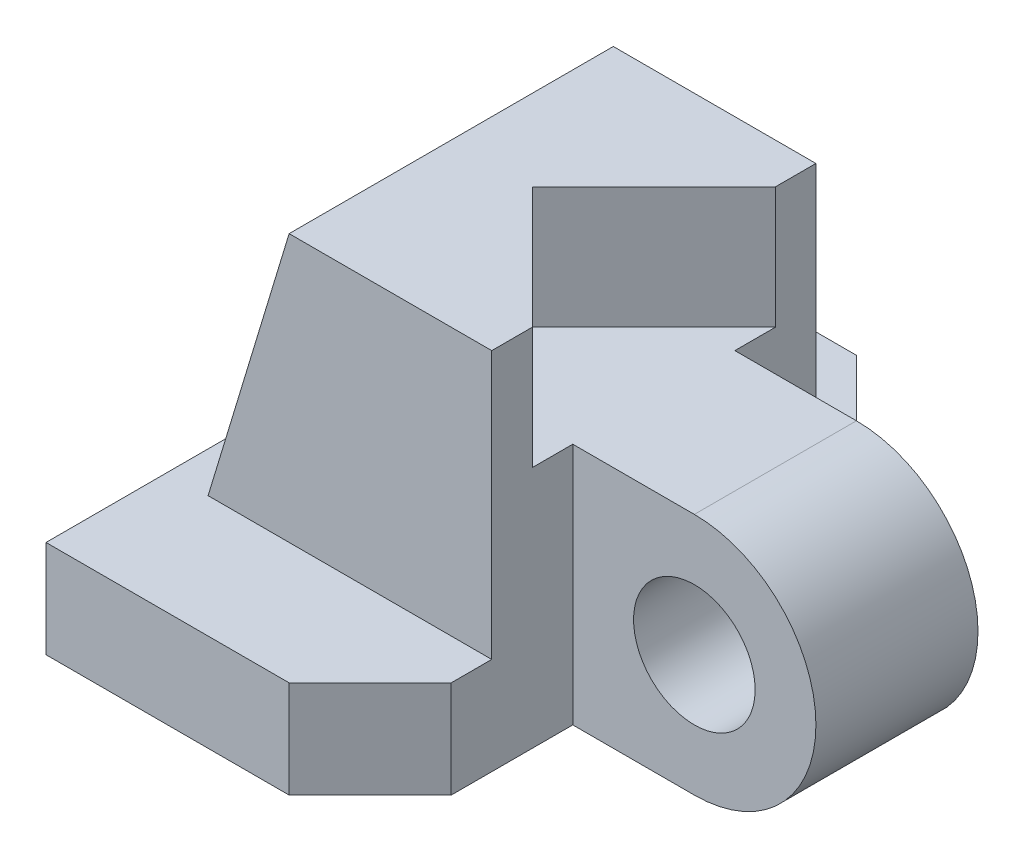
ISO-10303-21;
HEADER;
FILE_DESCRIPTION(('STEP AP214'),'2;1');
FILE_NAME('part.step','',(''),(''),'','','');
FILE_SCHEMA(('AUTOMOTIVE_DESIGN { 1 0 10303 214 1 1 1 1 }'));
ENDSEC;
DATA;
#1=APPLICATION_CONTEXT('core data for automotive mechanical design processes');
#2=APPLICATION_PROTOCOL_DEFINITION('international standard','automotive_design',2000,#1);
#3=PRODUCT_CONTEXT('',#1,'mechanical');
#4=PRODUCT('Part','Part','',(#3));
#5=PRODUCT_RELATED_PRODUCT_CATEGORY('part','',(#4));
#6=PRODUCT_DEFINITION_FORMATION('','',#4);
#7=PRODUCT_DEFINITION_CONTEXT('part definition',#1,'design');
#8=PRODUCT_DEFINITION('design','',#6,#7);
#9=PRODUCT_DEFINITION_SHAPE('','',#8);
#10=(LENGTH_UNIT() NAMED_UNIT(*) SI_UNIT(.MILLI.,.METRE.));
#11=(NAMED_UNIT(*) PLANE_ANGLE_UNIT() SI_UNIT($,.RADIAN.));
#12=(NAMED_UNIT(*) SI_UNIT($,.STERADIAN.) SOLID_ANGLE_UNIT());
#13=UNCERTAINTY_MEASURE_WITH_UNIT(LENGTH_MEASURE(1.E-05),#10,'distance_accuracy_value','');
#14=(GEOMETRIC_REPRESENTATION_CONTEXT(3) GLOBAL_UNCERTAINTY_ASSIGNED_CONTEXT((#13)) GLOBAL_UNIT_ASSIGNED_CONTEXT((#10,
#11,#12)) REPRESENTATION_CONTEXT('',''));
#15=CARTESIAN_POINT('',(0.,0.,0.));
#16=DIRECTION('',(0.,0.,1.));
#17=DIRECTION('',(1.,0.,0.));
#18=AXIS2_PLACEMENT_3D('',#15,#16,#17);
#19=CARTESIAN_POINT('',(-15.,0.,35.));
#20=DIRECTION('',(1.,0.,0.));
#21=DIRECTION('',(0.,1.,0.));
#22=AXIS2_PLACEMENT_3D('',#19,#20,#21);
#23=PLANE('',#22);
#24=DIRECTION('',(0.,0.,-1.));
#25=VECTOR('',#24,1.);
#26=CARTESIAN_POINT('',(-15.,15.,-15.));
#27=LINE('',#26,#25);
#28=CARTESIAN_POINT('',(-15.,15.,15.));
#29=VERTEX_POINT('',#28);
#30=CARTESIAN_POINT('',(-15.,15.,10.));
#31=VERTEX_POINT('',#30);
#32=EDGE_CURVE('E209',#29,#31,#27,.T.);
#33=ORIENTED_EDGE('',*,*,#32,.F.);
#34=DIRECTION('',(0.,1.,0.));
#35=VECTOR('',#34,1.);
#36=CARTESIAN_POINT('',(-15.,-18.5410196624968,15.));
#37=LINE('',#36,#35);
#38=CARTESIAN_POINT('',(-15.,30.,15.));
#39=VERTEX_POINT('',#38);
#40=EDGE_CURVE('E195',#29,#39,#37,.T.);
#41=ORIENTED_EDGE('',*,*,#40,.T.);
#42=DIRECTION('',(0.,0.,-1.));
#43=VECTOR('',#42,1.);
#44=CARTESIAN_POINT('',(-15.,30.,20.));
#45=LINE('',#44,#43);
#46=CARTESIAN_POINT('',(-15.,30.,20.));
#47=VERTEX_POINT('',#46);
#48=EDGE_CURVE('E245',#47,#39,#45,.T.);
#49=ORIENTED_EDGE('',*,*,#48,.F.);
#50=DIRECTION('',(0.,1.,0.));
#51=VECTOR('',#50,1.);
#52=CARTESIAN_POINT('',(-15.,0.,20.));
#53=LINE('',#52,#51);
#54=CARTESIAN_POINT('',(-15.,-3.,20.));
#55=VERTEX_POINT('',#54);
#56=EDGE_CURVE('E216',#55,#47,#53,.T.);
#57=ORIENTED_EDGE('',*,*,#56,.F.);
#58=DIRECTION('',(0.,0.,-1.));
#59=VECTOR('',#58,1.);
#60=CARTESIAN_POINT('',(-15.,-3.,35.));
#61=LINE('',#60,#59);
#62=CARTESIAN_POINT('',(-15.,-3.,25.));
#63=VERTEX_POINT('',#62);
#64=EDGE_CURVE('E267',#63,#55,#61,.T.);
#65=ORIENTED_EDGE('',*,*,#64,.F.);
#66=DIRECTION('',(0.,-1.,0.));
#67=VECTOR('',#66,1.);
#68=CARTESIAN_POINT('',(-15.,0.,25.));
#69=LINE('',#68,#67);
#70=CARTESIAN_POINT('',(-15.,-15.,25.));
#71=VERTEX_POINT('',#70);
#72=EDGE_CURVE('E313',#63,#71,#69,.T.);
#73=ORIENTED_EDGE('',*,*,#72,.T.);
#74=DIRECTION('',(0.,0.,-1.));
#75=VECTOR('',#74,1.);
#76=CARTESIAN_POINT('',(-15.,-15.,35.));
#77=LINE('',#76,#75);
#78=CARTESIAN_POINT('',(-15.,-15.,10.));
#79=VERTEX_POINT('',#78);
#80=EDGE_CURVE('E265',#71,#79,#77,.T.);
#81=ORIENTED_EDGE('',*,*,#80,.T.);
#82=DIRECTION('',(0.,1.,0.));
#83=VECTOR('',#82,1.);
#84=CARTESIAN_POINT('',(-15.,0.,10.));
#85=LINE('',#84,#83);
#86=EDGE_CURVE('E282',#79,#31,#85,.T.);
#87=ORIENTED_EDGE('',*,*,#86,.T.);
#88=EDGE_LOOP('',(#33,#41,#49,#57,#65,#73,#81,#87));
#89=FACE_BOUND('',#88,.T.);
#90=ADVANCED_FACE('F70',(#89),#23,.T.);
#91=CARTESIAN_POINT('',(0.,30.,20.));
#92=DIRECTION('',(0.,-1.,0.));
#93=DIRECTION('',(1.,0.,0.));
#94=AXIS2_PLACEMENT_3D('',#91,#92,#93);
#95=PLANE('',#94);
#96=DIRECTION('',(-0.707106781186547,0.,0.707106781186548));
#97=VECTOR('',#96,1.);
#98=CARTESIAN_POINT('',(-30.,30.,0.));
#99=LINE('',#98,#97);
#100=CARTESIAN_POINT('',(-15.,30.,-15.));
#101=VERTEX_POINT('',#100);
#102=CARTESIAN_POINT('',(-30.,30.,0.));
#103=VERTEX_POINT('',#102);
#104=EDGE_CURVE('E82',#101,#103,#99,.T.);
#105=ORIENTED_EDGE('',*,*,#104,.F.);
#106=CARTESIAN_POINT('',(-15.,30.,-20.));
#107=VERTEX_POINT('',#106);
#108=EDGE_CURVE('E243',#101,#107,#45,.T.);
#109=ORIENTED_EDGE('',*,*,#108,.T.);
#110=DIRECTION('',(-1.,0.,0.));
#111=VECTOR('',#110,1.);
#112=CARTESIAN_POINT('',(0.,30.,-20.));
#113=LINE('',#112,#111);
#114=CARTESIAN_POINT('',(-40.,30.,-20.));
#115=VERTEX_POINT('',#114);
#116=EDGE_CURVE('E231',#107,#115,#113,.T.);
#117=ORIENTED_EDGE('',*,*,#116,.T.);
#118=DIRECTION('',(0.,0.,-1.));
#119=VECTOR('',#118,1.);
#120=CARTESIAN_POINT('',(-40.,30.,20.));
#121=LINE('',#120,#119);
#122=CARTESIAN_POINT('',(-40.,30.,20.));
#123=VERTEX_POINT('',#122);
#124=EDGE_CURVE('E239',#123,#115,#121,.T.);
#125=ORIENTED_EDGE('',*,*,#124,.F.);
#126=DIRECTION('',(-1.,0.,0.));
#127=VECTOR('',#126,1.);
#128=CARTESIAN_POINT('',(0.,30.,20.));
#129=LINE('',#128,#127);
#130=EDGE_CURVE('E218',#47,#123,#129,.T.);
#131=ORIENTED_EDGE('',*,*,#130,.F.);
#132=ORIENTED_EDGE('',*,*,#48,.T.);
#133=DIRECTION('',(0.707106781186547,0.,0.707106781186548));
#134=VECTOR('',#133,1.);
#135=CARTESIAN_POINT('',(-15.,30.,15.));
#136=LINE('',#135,#134);
#137=EDGE_CURVE('E202',#103,#39,#136,.T.);
#138=ORIENTED_EDGE('',*,*,#137,.F.);
#139=EDGE_LOOP('',(#105,#109,#117,#125,#131,#132,#138));
#140=FACE_BOUND('',#139,.T.);
#141=ADVANCED_FACE('F366',(#140),#95,.F.);
#142=CARTESIAN_POINT('',(0.,-3.,35.));
#143=DIRECTION('',(0.,1.,0.));
#144=DIRECTION('',(-1.,0.,0.));
#145=AXIS2_PLACEMENT_3D('',#142,#143,#144);
#146=PLANE('',#145);
#147=CARTESIAN_POINT('',(-15.,-3.,-20.));
#148=VERTEX_POINT('',#147);
#149=CARTESIAN_POINT('',(-15.,-3.,-25.));
#150=VERTEX_POINT('',#149);
#151=EDGE_CURVE('E268',#148,#150,#61,.T.);
#152=ORIENTED_EDGE('',*,*,#151,.T.);
#153=DIRECTION('',(-0.707106781186547,0.,-0.707106781186548));
#154=VECTOR('',#153,1.);
#155=CARTESIAN_POINT('',(22.5,-3.,12.5));
#156=LINE('',#155,#154);
#157=CARTESIAN_POINT('',(-25.,-3.,-35.));
#158=VERTEX_POINT('',#157);
#159=EDGE_CURVE('E78',#150,#158,#156,.T.);
#160=ORIENTED_EDGE('',*,*,#159,.T.);
#161=DIRECTION('',(1.,0.,0.));
#162=VECTOR('',#161,1.);
#163=CARTESIAN_POINT('',(0.,-3.,-35.));
#164=LINE('',#163,#162);
#165=CARTESIAN_POINT('',(-55.,-3.,-35.));
#166=VERTEX_POINT('',#165);
#167=EDGE_CURVE('E244',#166,#158,#164,.T.);
#168=ORIENTED_EDGE('',*,*,#167,.F.);
#169=DIRECTION('',(0.,0.,-1.));
#170=VECTOR('',#169,1.);
#171=CARTESIAN_POINT('',(-55.,-3.,35.));
#172=LINE('',#171,#170);
#173=CARTESIAN_POINT('',(-55.,-3.,35.));
#174=VERTEX_POINT('',#173);
#175=EDGE_CURVE('E266',#174,#166,#172,.T.);
#176=ORIENTED_EDGE('',*,*,#175,.F.);
#177=DIRECTION('',(1.,0.,0.));
#178=VECTOR('',#177,1.);
#179=CARTESIAN_POINT('',(0.,-3.,35.));
#180=LINE('',#179,#178);
#181=CARTESIAN_POINT('',(-25.,-3.,35.));
#182=VERTEX_POINT('',#181);
#183=EDGE_CURVE('E246',#174,#182,#180,.T.);
#184=ORIENTED_EDGE('',*,*,#183,.T.);
#185=DIRECTION('',(-0.707106781186547,0.,0.707106781186548));
#186=VECTOR('',#185,1.);
#187=CARTESIAN_POINT('',(-12.5,-3.,22.5));
#188=LINE('',#187,#186);
#189=EDGE_CURVE('E316',#182,#63,#188,.F.);
#190=ORIENTED_EDGE('',*,*,#189,.T.);
#191=ORIENTED_EDGE('',*,*,#64,.T.);
#192=DIRECTION('',(1.,0.,0.));
#193=VECTOR('',#192,1.);
#194=CARTESIAN_POINT('',(0.,-3.,20.));
#195=LINE('',#194,#193);
#196=CARTESIAN_POINT('',(-50.,-3.,20.));
#197=VERTEX_POINT('',#196);
#198=EDGE_CURVE('E223',#197,#55,#195,.T.);
#199=ORIENTED_EDGE('',*,*,#198,.F.);
#200=DIRECTION('',(0.,0.,-1.));
#201=VECTOR('',#200,1.);
#202=CARTESIAN_POINT('',(-50.,-3.,20.));
#203=LINE('',#202,#201);
#204=CARTESIAN_POINT('',(-50.,-3.,-20.));
#205=VERTEX_POINT('',#204);
#206=EDGE_CURVE('E226',#197,#205,#203,.T.);
#207=ORIENTED_EDGE('',*,*,#206,.T.);
#208=DIRECTION('',(1.,0.,0.));
#209=VECTOR('',#208,1.);
#210=CARTESIAN_POINT('',(0.,-3.,-20.));
#211=LINE('',#210,#209);
#212=EDGE_CURVE('E219',#205,#148,#211,.T.);
#213=ORIENTED_EDGE('',*,*,#212,.T.);
#214=EDGE_LOOP('',(#152,#160,#168,#176,#184,#190,#191,#199,#207,#213));
#215=FACE_BOUND('',#214,.T.);
#216=ADVANCED_FACE('F321',(#215),#146,.T.);
#217=CARTESIAN_POINT('',(0.,-15.,10.));
#218=DIRECTION('',(0.,1.,0.));
#219=DIRECTION('',(-1.,0.,0.));
#220=AXIS2_PLACEMENT_3D('',#217,#218,#219);
#221=PLANE('',#220);
#222=DIRECTION('',(1.,0.,0.));
#223=VECTOR('',#222,1.);
#224=CARTESIAN_POINT('',(0.,-15.,-35.));
#225=LINE('',#224,#223);
#226=CARTESIAN_POINT('',(-55.,-15.,-35.));
#227=VERTEX_POINT('',#226);
#228=CARTESIAN_POINT('',(-25.,-15.,-35.));
#229=VERTEX_POINT('',#228);
#230=EDGE_CURVE('E248',#227,#229,#225,.T.);
#231=ORIENTED_EDGE('',*,*,#230,.T.);
#232=DIRECTION('',(0.707106781186547,0.,0.707106781186548));
#233=VECTOR('',#232,1.);
#234=CARTESIAN_POINT('',(-25.,-15.,-35.));
#235=LINE('',#234,#233);
#236=CARTESIAN_POINT('',(-15.,-15.,-25.));
#237=VERTEX_POINT('',#236);
#238=EDGE_CURVE('E310',#229,#237,#235,.T.);
#239=ORIENTED_EDGE('',*,*,#238,.T.);
#240=CARTESIAN_POINT('',(-15.,-15.,-10.));
#241=VERTEX_POINT('',#240);
#242=EDGE_CURVE('E255',#241,#237,#77,.T.);
#243=ORIENTED_EDGE('',*,*,#242,.F.);
#244=DIRECTION('',(1.,0.,0.));
#245=VECTOR('',#244,1.);
#246=CARTESIAN_POINT('',(0.,-15.,-10.));
#247=LINE('',#246,#245);
#248=CARTESIAN_POINT('',(1.57116657546902E-13,-15.,-10.));
#249=VERTEX_POINT('',#248);
#250=EDGE_CURVE('E289',#241,#249,#247,.T.);
#251=ORIENTED_EDGE('',*,*,#250,.T.);
#252=DIRECTION('',(0.,0.,-1.));
#253=VECTOR('',#252,1.);
#254=CARTESIAN_POINT('',(1.57116657546902E-13,-15.,10.));
#255=LINE('',#254,#253);
#256=CARTESIAN_POINT('',(1.57116657546902E-13,-15.,10.));
#257=VERTEX_POINT('',#256);
#258=EDGE_CURVE('E301',#257,#249,#255,.T.);
#259=ORIENTED_EDGE('',*,*,#258,.F.);
#260=DIRECTION('',(1.,0.,0.));
#261=VECTOR('',#260,1.);
#262=CARTESIAN_POINT('',(0.,-15.,10.));
#263=LINE('',#262,#261);
#264=EDGE_CURVE('E274',#79,#257,#263,.T.);
#265=ORIENTED_EDGE('',*,*,#264,.F.);
#266=ORIENTED_EDGE('',*,*,#80,.F.);
#267=DIRECTION('',(0.707106781186547,0.,-0.707106781186548));
#268=VECTOR('',#267,1.);
#269=CARTESIAN_POINT('',(-15.,-15.,25.));
#270=LINE('',#269,#268);
#271=CARTESIAN_POINT('',(-25.,-15.,35.));
#272=VERTEX_POINT('',#271);
#273=EDGE_CURVE('E307',#71,#272,#270,.F.);
#274=ORIENTED_EDGE('',*,*,#273,.T.);
#275=DIRECTION('',(1.,0.,0.));
#276=VECTOR('',#275,1.);
#277=CARTESIAN_POINT('',(0.,-15.,35.));
#278=LINE('',#277,#276);
#279=CARTESIAN_POINT('',(-55.,-15.,35.));
#280=VERTEX_POINT('',#279);
#281=EDGE_CURVE('E252',#280,#272,#278,.T.);
#282=ORIENTED_EDGE('',*,*,#281,.F.);
#283=DIRECTION('',(0.,0.,-1.));
#284=VECTOR('',#283,1.);
#285=CARTESIAN_POINT('',(-55.,-15.,35.));
#286=LINE('',#285,#284);
#287=EDGE_CURVE('E262',#280,#227,#286,.T.);
#288=ORIENTED_EDGE('',*,*,#287,.T.);
#289=EDGE_LOOP('',(#231,#239,#243,#251,#259,#265,#266,#274,#282,#288));
#290=FACE_BOUND('',#289,.T.);
#291=ADVANCED_FACE('F331',(#290),#221,.F.);
#292=CARTESIAN_POINT('',(0.,0.,10.));
#293=DIRECTION('',(0.,0.,-1.));
#294=DIRECTION('',(-1.,0.,0.));
#295=AXIS2_PLACEMENT_3D('',#292,#293,#294);
#296=CYLINDRICAL_SURFACE('',#295,15.);
#297=CARTESIAN_POINT('',(0.,0.,-10.));
#298=DIRECTION('',(0.,0.,1.));
#299=DIRECTION('',(1.,0.,0.));
#300=AXIS2_PLACEMENT_3D('',#297,#298,#299);
#301=CIRCLE('',#300,15.);
#302=CARTESIAN_POINT('',(0.,15.,-10.));
#303=VERTEX_POINT('',#302);
#304=EDGE_CURVE('E291',#249,#303,#301,.T.);
#305=ORIENTED_EDGE('',*,*,#304,.T.);
#306=DIRECTION('',(0.,0.,-1.));
#307=VECTOR('',#306,1.);
#308=CARTESIAN_POINT('',(0.,15.,10.));
#309=LINE('',#308,#307);
#310=CARTESIAN_POINT('',(0.,15.,10.));
#311=VERTEX_POINT('',#310);
#312=EDGE_CURVE('E290',#311,#303,#309,.T.);
#313=ORIENTED_EDGE('',*,*,#312,.F.);
#314=CARTESIAN_POINT('',(0.,0.,10.));
#315=DIRECTION('',(0.,0.,1.));
#316=DIRECTION('',(1.,0.,0.));
#317=AXIS2_PLACEMENT_3D('',#314,#315,#316);
#318=CIRCLE('',#317,15.);
#319=EDGE_CURVE('E276',#257,#311,#318,.T.);
#320=ORIENTED_EDGE('',*,*,#319,.F.);
#321=ORIENTED_EDGE('',*,*,#258,.T.);
#322=EDGE_LOOP('',(#305,#313,#320,#321));
#323=FACE_BOUND('',#322,.T.);
#324=ADVANCED_FACE('F343',(#323),#296,.T.);
#325=CARTESIAN_POINT('',(0.,15.,10.));
#326=DIRECTION('',(0.,-1.,0.));
#327=DIRECTION('',(1.,0.,0.));
#328=AXIS2_PLACEMENT_3D('',#325,#326,#327);
#329=PLANE('',#328);
#330=DIRECTION('',(-1.,0.,0.));
#331=VECTOR('',#330,1.);
#332=CARTESIAN_POINT('',(0.,15.,-10.));
#333=LINE('',#332,#331);
#334=CARTESIAN_POINT('',(-15.,15.,-10.));
#335=VERTEX_POINT('',#334);
#336=EDGE_CURVE('E293',#303,#335,#333,.T.);
#337=ORIENTED_EDGE('',*,*,#336,.T.);
#338=CARTESIAN_POINT('',(-15.,15.,-15.));
#339=VERTEX_POINT('',#338);
#340=EDGE_CURVE('E204',#335,#339,#27,.T.);
#341=ORIENTED_EDGE('',*,*,#340,.T.);
#342=DIRECTION('',(-0.707106781186547,0.,0.707106781186548));
#343=VECTOR('',#342,1.);
#344=CARTESIAN_POINT('',(-30.,15.,0.));
#345=LINE('',#344,#343);
#346=CARTESIAN_POINT('',(-30.,15.,0.));
#347=VERTEX_POINT('',#346);
#348=EDGE_CURVE('E200',#339,#347,#345,.T.);
#349=ORIENTED_EDGE('',*,*,#348,.T.);
#350=DIRECTION('',(0.707106781186547,0.,0.707106781186548));
#351=VECTOR('',#350,1.);
#352=CARTESIAN_POINT('',(-15.,15.,15.));
#353=LINE('',#352,#351);
#354=EDGE_CURVE('E190',#347,#29,#353,.T.);
#355=ORIENTED_EDGE('',*,*,#354,.T.);
#356=ORIENTED_EDGE('',*,*,#32,.T.);
#357=DIRECTION('',(-1.,0.,0.));
#358=VECTOR('',#357,1.);
#359=CARTESIAN_POINT('',(0.,15.,10.));
#360=LINE('',#359,#358);
#361=EDGE_CURVE('E283',#311,#31,#360,.T.);
#362=ORIENTED_EDGE('',*,*,#361,.F.);
#363=ORIENTED_EDGE('',*,*,#312,.T.);
#364=EDGE_LOOP('',(#337,#341,#349,#355,#356,#362,#363));
#365=FACE_BOUND('',#364,.T.);
#366=ADVANCED_FACE('F201',(#365),#329,.F.);
#367=CARTESIAN_POINT('',(0.,0.,10.));
#368=DIRECTION('',(0.,0.,-1.));
#369=DIRECTION('',(-1.,0.,0.));
#370=AXIS2_PLACEMENT_3D('',#367,#368,#369);
#371=CYLINDRICAL_SURFACE('',#370,7.5);
#372=CARTESIAN_POINT('',(0.,0.,10.));
#373=DIRECTION('',(0.,0.,1.));
#374=DIRECTION('',(1.,0.,0.));
#375=AXIS2_PLACEMENT_3D('',#372,#373,#374);
#376=CIRCLE('',#375,7.5);
#377=CARTESIAN_POINT('',(7.5,0.,10.));
#378=VERTEX_POINT('',#377);
#379=EDGE_CURVE('E275',#378,#378,#376,.T.);
#380=ORIENTED_EDGE('',*,*,#379,.T.);
#381=EDGE_LOOP('',(#380));
#382=FACE_BOUND('',#381,.T.);
#383=CARTESIAN_POINT('',(0.,0.,-10.));
#384=DIRECTION('',(0.,0.,1.));
#385=DIRECTION('',(1.,0.,0.));
#386=AXIS2_PLACEMENT_3D('',#383,#384,#385);
#387=CIRCLE('',#386,7.5);
#388=CARTESIAN_POINT('',(7.5,0.,-10.));
#389=VERTEX_POINT('',#388);
#390=EDGE_CURVE('E271',#389,#389,#387,.T.);
#391=ORIENTED_EDGE('',*,*,#390,.F.);
#392=EDGE_LOOP('',(#391));
#393=FACE_BOUND('',#392,.T.);
#394=ADVANCED_FACE('F407',(#382,#393),#371,.F.);
#395=CARTESIAN_POINT('',(0.,0.,10.));
#396=DIRECTION('',(0.,0.,1.));
#397=DIRECTION('',(1.,0.,0.));
#398=AXIS2_PLACEMENT_3D('',#395,#396,#397);
#399=PLANE('',#398);
#400=ORIENTED_EDGE('',*,*,#379,.F.);
#401=EDGE_LOOP('',(#400));
#402=FACE_BOUND('',#401,.T.);
#403=ORIENTED_EDGE('',*,*,#264,.T.);
#404=ORIENTED_EDGE('',*,*,#319,.T.);
#405=ORIENTED_EDGE('',*,*,#361,.T.);
#406=ORIENTED_EDGE('',*,*,#86,.F.);
#407=EDGE_LOOP('',(#403,#404,#405,#406));
#408=FACE_BOUND('',#407,.T.);
#409=ADVANCED_FACE('F348',(#402,#408),#399,.T.);
#410=CARTESIAN_POINT('',(0.,0.,-10.));
#411=DIRECTION('',(0.,0.,1.));
#412=DIRECTION('',(1.,0.,0.));
#413=AXIS2_PLACEMENT_3D('',#410,#411,#412);
#414=PLANE('',#413);
#415=ORIENTED_EDGE('',*,*,#390,.T.);
#416=EDGE_LOOP('',(#415));
#417=FACE_BOUND('',#416,.T.);
#418=ORIENTED_EDGE('',*,*,#250,.F.);
#419=DIRECTION('',(0.,1.,0.));
#420=VECTOR('',#419,1.);
#421=CARTESIAN_POINT('',(-15.,0.,-10.));
#422=LINE('',#421,#420);
#423=EDGE_CURVE('E277',#241,#335,#422,.T.);
#424=ORIENTED_EDGE('',*,*,#423,.T.);
#425=ORIENTED_EDGE('',*,*,#336,.F.);
#426=ORIENTED_EDGE('',*,*,#304,.F.);
#427=EDGE_LOOP('',(#418,#424,#425,#426));
#428=FACE_BOUND('',#427,.T.);
#429=ADVANCED_FACE('F339',(#417,#428),#414,.F.);
#430=ORIENTED_EDGE('',*,*,#340,.F.);
#431=ORIENTED_EDGE('',*,*,#423,.F.);
#432=ORIENTED_EDGE('',*,*,#242,.T.);
#433=DIRECTION('',(0.,1.,0.));
#434=VECTOR('',#433,1.);
#435=CARTESIAN_POINT('',(-15.,-3.,-25.));
#436=LINE('',#435,#434);
#437=EDGE_CURVE('E314',#237,#150,#436,.T.);
#438=ORIENTED_EDGE('',*,*,#437,.T.);
#439=ORIENTED_EDGE('',*,*,#151,.F.);
#440=DIRECTION('',(0.,1.,0.));
#441=VECTOR('',#440,1.);
#442=CARTESIAN_POINT('',(-15.,0.,-20.));
#443=LINE('',#442,#441);
#444=EDGE_CURVE('E214',#148,#107,#443,.T.);
#445=ORIENTED_EDGE('',*,*,#444,.T.);
#446=ORIENTED_EDGE('',*,*,#108,.F.);
#447=DIRECTION('',(0.,1.,0.));
#448=VECTOR('',#447,1.);
#449=CARTESIAN_POINT('',(-15.,-18.5410196624968,-15.));
#450=LINE('',#449,#448);
#451=EDGE_CURVE('E211',#339,#101,#450,.T.);
#452=ORIENTED_EDGE('',*,*,#451,.F.);
#453=EDGE_LOOP('',(#430,#431,#432,#438,#439,#445,#446,#452));
#454=FACE_BOUND('',#453,.T.);
#455=ADVANCED_FACE('F340',(#454),#23,.T.);
#456=CARTESIAN_POINT('',(0.,0.,-35.));
#457=DIRECTION('',(0.,0.,1.));
#458=DIRECTION('',(1.,0.,0.));
#459=AXIS2_PLACEMENT_3D('',#456,#457,#458);
#460=PLANE('',#459);
#461=ORIENTED_EDGE('',*,*,#167,.T.);
#462=DIRECTION('',(0.,-1.,0.));
#463=VECTOR('',#462,1.);
#464=CARTESIAN_POINT('',(-25.,-15.,-35.));
#465=LINE('',#464,#463);
#466=EDGE_CURVE('E303',#158,#229,#465,.T.);
#467=ORIENTED_EDGE('',*,*,#466,.T.);
#468=ORIENTED_EDGE('',*,*,#230,.F.);
#469=DIRECTION('',(0.,1.,0.));
#470=VECTOR('',#469,1.);
#471=CARTESIAN_POINT('',(-55.,0.,-35.));
#472=LINE('',#471,#470);
#473=EDGE_CURVE('E260',#227,#166,#472,.T.);
#474=ORIENTED_EDGE('',*,*,#473,.T.);
#475=EDGE_LOOP('',(#461,#467,#468,#474));
#476=FACE_BOUND('',#475,.T.);
#477=ADVANCED_FACE('F330',(#476),#460,.F.);
#478=CARTESIAN_POINT('',(-55.,0.,35.));
#479=DIRECTION('',(-1.,0.,0.));
#480=DIRECTION('',(0.,0.,1.));
#481=AXIS2_PLACEMENT_3D('',#478,#479,#480);
#482=PLANE('',#481);
#483=ORIENTED_EDGE('',*,*,#473,.F.);
#484=ORIENTED_EDGE('',*,*,#287,.F.);
#485=DIRECTION('',(0.,1.,0.));
#486=VECTOR('',#485,1.);
#487=CARTESIAN_POINT('',(-55.,0.,35.));
#488=LINE('',#487,#486);
#489=EDGE_CURVE('E247',#280,#174,#488,.T.);
#490=ORIENTED_EDGE('',*,*,#489,.T.);
#491=ORIENTED_EDGE('',*,*,#175,.T.);
#492=EDGE_LOOP('',(#483,#484,#490,#491));
#493=FACE_BOUND('',#492,.T.);
#494=ADVANCED_FACE('F363',(#493),#482,.T.);
#495=CARTESIAN_POINT('',(0.,0.,35.));
#496=DIRECTION('',(0.,0.,1.));
#497=DIRECTION('',(1.,0.,0.));
#498=AXIS2_PLACEMENT_3D('',#495,#496,#497);
#499=PLANE('',#498);
#500=ORIENTED_EDGE('',*,*,#281,.T.);
#501=DIRECTION('',(0.,1.,0.));
#502=VECTOR('',#501,1.);
#503=CARTESIAN_POINT('',(-25.,0.,35.));
#504=LINE('',#503,#502);
#505=EDGE_CURVE('E12',#272,#182,#504,.T.);
#506=ORIENTED_EDGE('',*,*,#505,.T.);
#507=ORIENTED_EDGE('',*,*,#183,.F.);
#508=ORIENTED_EDGE('',*,*,#489,.F.);
#509=EDGE_LOOP('',(#500,#506,#507,#508));
#510=FACE_BOUND('',#509,.T.);
#511=ADVANCED_FACE('F358',(#510),#499,.T.);
#512=CARTESIAN_POINT('',(-44.9621530698066,13.6248948696384,20.));
#513=DIRECTION('',(-0.957024404433474,0.290007395282871,0.));
#514=DIRECTION('',(-0.290007395282871,-0.957024404433474,0.));
#515=AXIS2_PLACEMENT_3D('',#512,#513,#514);
#516=PLANE('',#515);
#517=DIRECTION('',(0.290007395282871,0.957024404433474,0.));
#518=VECTOR('',#517,1.);
#519=CARTESIAN_POINT('',(-44.9621530698066,13.6248948696384,-20.));
#520=LINE('',#519,#518);
#521=EDGE_CURVE('E233',#205,#115,#520,.T.);
#522=ORIENTED_EDGE('',*,*,#521,.F.);
#523=ORIENTED_EDGE('',*,*,#206,.F.);
#524=DIRECTION('',(0.290007395282871,0.957024404433474,0.));
#525=VECTOR('',#524,1.);
#526=CARTESIAN_POINT('',(-44.9621530698066,13.6248948696384,20.));
#527=LINE('',#526,#525);
#528=EDGE_CURVE('E225',#197,#123,#527,.T.);
#529=ORIENTED_EDGE('',*,*,#528,.T.);
#530=ORIENTED_EDGE('',*,*,#124,.T.);
#531=EDGE_LOOP('',(#522,#523,#529,#530));
#532=FACE_BOUND('',#531,.T.);
#533=ADVANCED_FACE('F373',(#532),#516,.T.);
#534=CARTESIAN_POINT('',(0.,0.,20.));
#535=DIRECTION('',(0.,0.,1.));
#536=DIRECTION('',(1.,0.,0.));
#537=AXIS2_PLACEMENT_3D('',#534,#535,#536);
#538=PLANE('',#537);
#539=ORIENTED_EDGE('',*,*,#56,.T.);
#540=ORIENTED_EDGE('',*,*,#130,.T.);
#541=ORIENTED_EDGE('',*,*,#528,.F.);
#542=ORIENTED_EDGE('',*,*,#198,.T.);
#543=EDGE_LOOP('',(#539,#540,#541,#542));
#544=FACE_BOUND('',#543,.T.);
#545=ADVANCED_FACE('F364',(#544),#538,.T.);
#546=CARTESIAN_POINT('',(0.,0.,-20.));
#547=DIRECTION('',(0.,0.,1.));
#548=DIRECTION('',(1.,0.,0.));
#549=AXIS2_PLACEMENT_3D('',#546,#547,#548);
#550=PLANE('',#549);
#551=ORIENTED_EDGE('',*,*,#444,.F.);
#552=ORIENTED_EDGE('',*,*,#212,.F.);
#553=ORIENTED_EDGE('',*,*,#521,.T.);
#554=ORIENTED_EDGE('',*,*,#116,.F.);
#555=EDGE_LOOP('',(#551,#552,#553,#554));
#556=FACE_BOUND('',#555,.T.);
#557=ADVANCED_FACE('F380',(#556),#550,.F.);
#558=CARTESIAN_POINT('',(-25.,0.,-35.));
#559=DIRECTION('',(0.707106781186548,0.,-0.707106781186547));
#560=DIRECTION('',(0.,1.,0.));
#561=AXIS2_PLACEMENT_3D('',#558,#559,#560);
#562=PLANE('',#561);
#563=ORIENTED_EDGE('',*,*,#159,.F.);
#564=ORIENTED_EDGE('',*,*,#437,.F.);
#565=ORIENTED_EDGE('',*,*,#238,.F.);
#566=ORIENTED_EDGE('',*,*,#466,.F.);
#567=EDGE_LOOP('',(#563,#564,#565,#566));
#568=FACE_BOUND('',#567,.T.);
#569=ADVANCED_FACE('F329',(#568),#562,.T.);
#570=CARTESIAN_POINT('',(-15.,0.,25.));
#571=DIRECTION('',(-0.707106781186548,0.,-0.707106781186547));
#572=DIRECTION('',(0.,-1.,0.));
#573=AXIS2_PLACEMENT_3D('',#570,#571,#572);
#574=PLANE('',#573);
#575=ORIENTED_EDGE('',*,*,#189,.F.);
#576=ORIENTED_EDGE('',*,*,#505,.F.);
#577=ORIENTED_EDGE('',*,*,#273,.F.);
#578=ORIENTED_EDGE('',*,*,#72,.F.);
#579=EDGE_LOOP('',(#575,#576,#577,#578));
#580=FACE_BOUND('',#579,.T.);
#581=ADVANCED_FACE('F69',(#580),#574,.F.);
#582=CARTESIAN_POINT('',(-30.,-18.5410196624969,0.));
#583=DIRECTION('',(-0.707106781186548,0.,-0.707106781186547));
#584=DIRECTION('',(-0.707106781186547,0.,0.707106781186548));
#585=AXIS2_PLACEMENT_3D('',#582,#583,#584);
#586=PLANE('',#585);
#587=ORIENTED_EDGE('',*,*,#451,.T.);
#588=ORIENTED_EDGE('',*,*,#104,.T.);
#589=DIRECTION('',(0.,1.,0.));
#590=VECTOR('',#589,1.);
#591=CARTESIAN_POINT('',(-30.,-18.5410196624969,0.));
#592=LINE('',#591,#590);
#593=EDGE_CURVE('E187',#347,#103,#592,.T.);
#594=ORIENTED_EDGE('',*,*,#593,.F.);
#595=ORIENTED_EDGE('',*,*,#348,.F.);
#596=EDGE_LOOP('',(#587,#588,#594,#595));
#597=FACE_BOUND('',#596,.T.);
#598=ADVANCED_FACE('F196',(#597),#586,.F.);
#599=CARTESIAN_POINT('',(-15.,-18.5410196624968,15.));
#600=DIRECTION('',(-0.707106781186548,0.,0.707106781186547));
#601=DIRECTION('',(0.707106781186547,0.,0.707106781186548));
#602=AXIS2_PLACEMENT_3D('',#599,#600,#601);
#603=PLANE('',#602);
#604=ORIENTED_EDGE('',*,*,#593,.T.);
#605=ORIENTED_EDGE('',*,*,#137,.T.);
#606=ORIENTED_EDGE('',*,*,#40,.F.);
#607=ORIENTED_EDGE('',*,*,#354,.F.);
#608=EDGE_LOOP('',(#604,#605,#606,#607));
#609=FACE_BOUND('',#608,.T.);
#610=ADVANCED_FACE('F186',(#609),#603,.F.);
#611=CLOSED_SHELL('',(#90,#141,#216,#291,#324,#366,#394,#409,#429,#455,#477,#494,#511,#533,#545,
#557,#569,#581,#598,#610));
#612=MANIFOLD_SOLID_BREP('B2',#611);
#613=ADVANCED_BREP_SHAPE_REPRESENTATION('',(#18,#612),#14);
#614=SHAPE_DEFINITION_REPRESENTATION(#9,#613);
ENDSEC;
END-ISO-10303-21;
